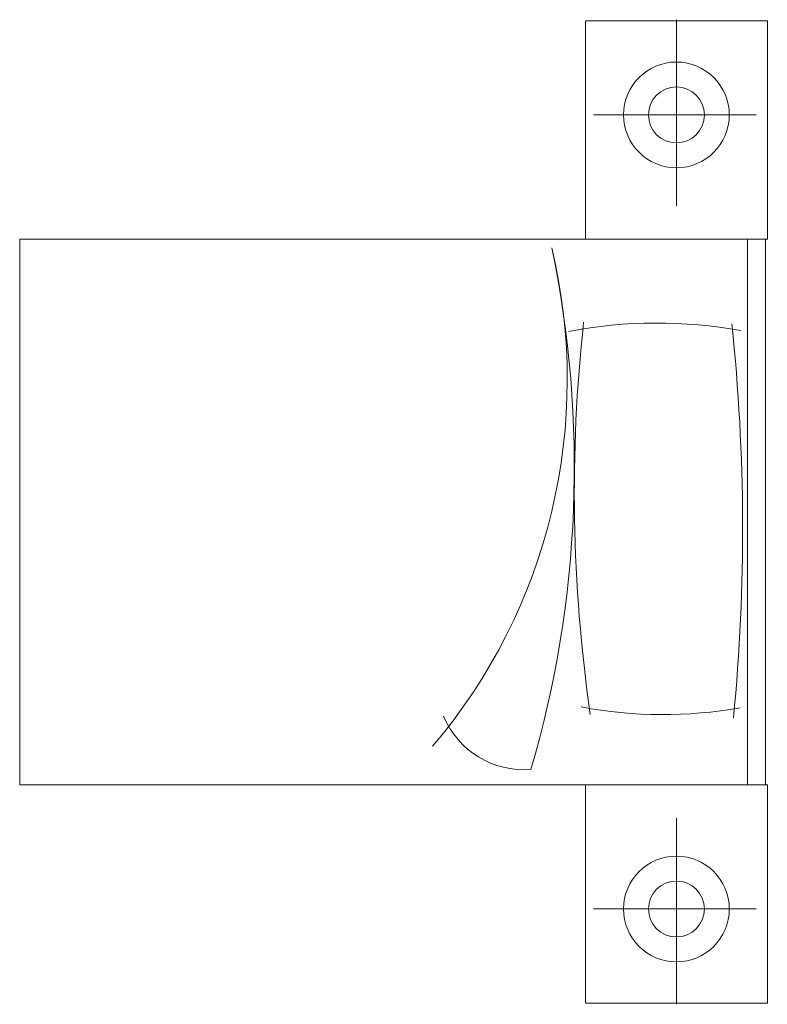
# Model space of a CAD drawing. Units: inches. Extents: x 20 to 32681, y 45 to 3082.
# Tile 4 of 5: x 222 to 333, y 1192 to 1339. Entities that reach past the tile are written whole.
import ezdxf

# ---------------------------------------------------------------- set-up
doc = ezdxf.new("R2010")
doc.units = ezdxf.units.IN
doc.header["$MEASUREMENT"] = 0
doc.layers.add('A-FURN', color=8, linetype='Continuous', lineweight=18)

# ---------------------------------------------------------------- blocks, each defined once
blk = doc.blocks.new('CVBN')
for p, q in [((89.36, 1192.66), (89.36, 1168.36)), ((170.36, 1192.66), (170.36, 1168.36)), ((70.94, 1179.16), (70.94, 1191.01)), ((89.36, 1081.69), (89.36, 1192.39)), ((89.36, 1192.39), (89.36, 1168.09)), ((170.36, 1192.39), (89.36, 1192.39)), ((170.36, 1081.69), (170.36, 1192.39)), ((170.36, 1192.39), (170.36, 1168.09)), ((170.36, 1192.39), (170.36, 1168.09)), ((188.79, 1179.16), (188.79, 1191.01)), ((170.36, 1189.69), (89.36, 1189.69)), ((70.94, 1179.16), (56.8, 1179.16)), ((70.94, 1179.16), (84.43, 1179.16)), ((70.94, 1179.16), (70.94, 1166.85)), ((188.79, 1179.16), (175.29, 1179.16)), ((188.79, 1179.16), (202.93, 1179.16)), ((188.79, 1179.16), (188.79, 1166.85)), ((170.36, 1081.69), (89.36, 1081.69))]:
    blk.add_line(p, q)
for points in [[(56.96, 1192.66), (56.96, 1165.66), (89.36, 1165.66), (89.36, 1192.66)], [(202.76, 1192.66), (202.76, 1165.66), (170.36, 1165.66), (170.36, 1192.66)]]:
    blk.add_lwpolyline(points, close=True)
for centre, radius in [((70.94, 1179.16), 7.85), ((188.79, 1179.16), 7.85), ((70.94, 1179.16), 4.15), ((188.79, 1179.16), 4.15)]:
    blk.add_circle(centre, radius)
for centre, radius, start, end in [((127.34, 900.05), 288.94, 83.953, 95.5626), ((165.23, 1177.16), 65.44, 169.9145, 190.6851), ((88.06, 1176.29), 69.84, 349.1761, 10.2706), ((132.8, 1394.24), 230.23, 261.7649, 276.2896), ((136.55, 1004.48), 159.53, 78.2462, 106.3473), ((149.51, 1078.87), 84.09, 76.5636, 130.3236), ((104.49, 1156.51), 12.88, 175.3269, 247.5588)]:
    blk.add_arc(centre, radius, start, end)

msp = doc.modelspace()

# ---------------------------------------------------------------- block references
at = {"layer": 'A-FURN', "xscale": -1, "rotation": 270}
msp.add_blockref('CVBN', (-860.02, 1135.7), dxfattribs=at)

doc.saveas('drawing.dxf')
